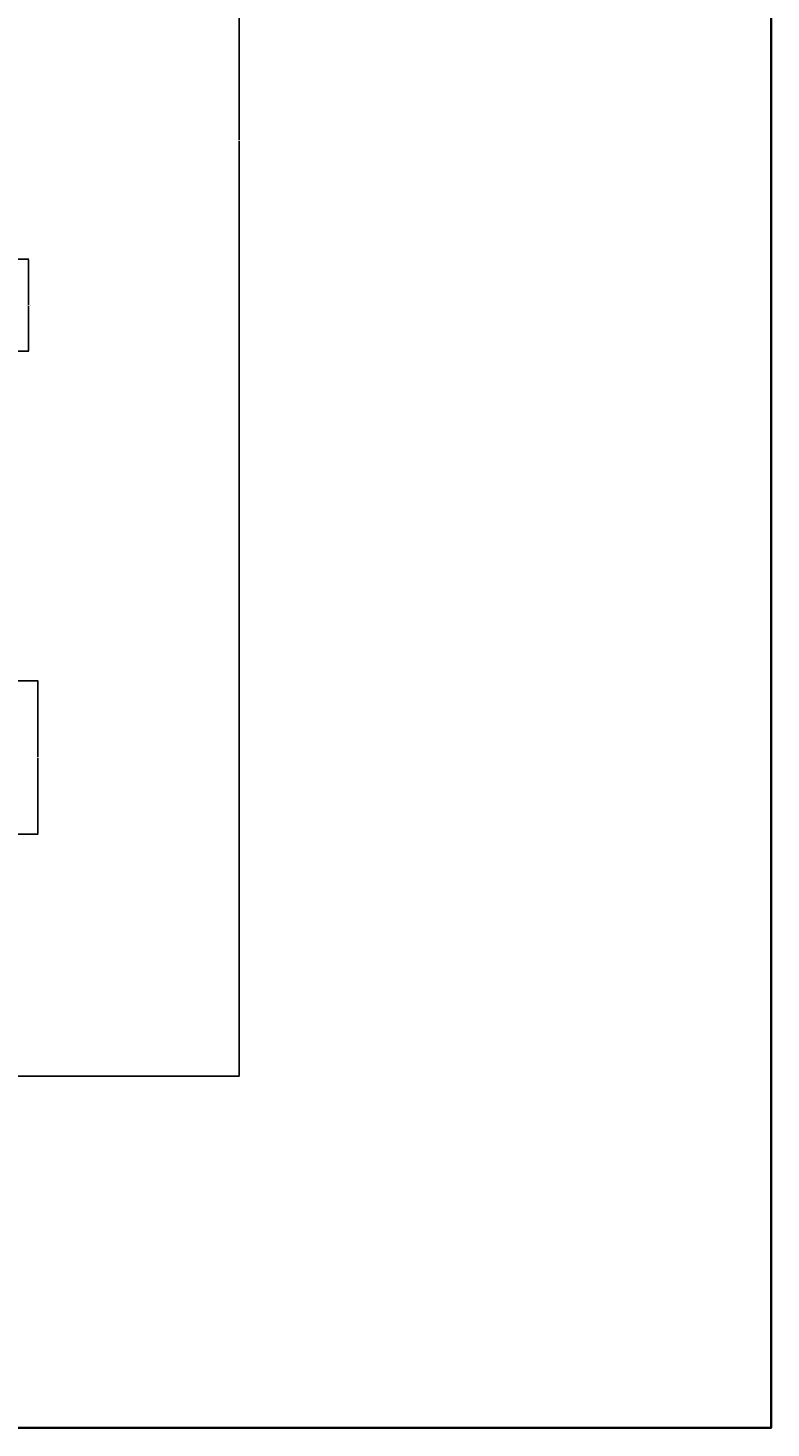
# Model space of a CAD drawing. Units: inches. Extents: x 1944 to 3454, y 1352 to 3055.
# Tile 12 of 17: x 3163 to 3454, y 1352 to 1900. Entities that reach past the tile are written whole.
import ezdxf

# ---------------------------------------------------------------- set-up
doc = ezdxf.new("R2010")
doc.units = ezdxf.units.IN
doc.layers.add('A-ANNO-DIMS', color=2, linetype='Continuous', lineweight=18)
doc.layers.add('A-ANNO-TTLB', color=7, linetype='Continuous', lineweight=35)
doc.styles.get("Standard").update_dxf_attribs({"font": 'arial.ttf'})
doc.dimstyles.get("Standard").update_dxf_attribs({"dimtxt": 0.18, "dimasz": 0.18, "dimexe": 0.18, "dimexo": 0.0625, "dimgap": 0.09, "dimtad": 0, "dimtih": 1, "dimtoh": 1, "dimdec": 4, "dimzin": 0, "dimdsep": 46, "dimtxsty": 'Standard', "dimcen": 0.09, "dimadec": 0, "dimazin": 0, "dimtfac": 1, "dimtdec": 4, "dimtofl": 0, "dimtmove": 0, "dimatfit": 3, "dimfxl": 1, "dimtolj": 1, "dimtzin": 0, "dimarcsym": 0})

# ---------------------------------------------------------------- blocks, each defined once
blk = doc.blocks.new('*D70')
at = {"layer": 'A-ANNO-DIMS', "color": 0, "lineweight": -2, "transparency": 16777216}
for p, q in [((3157.44, 1809.51), (3162.96, 1809.51)), ((3162.78, 1809.33), (3162.78, 1791.69)), ((3162.78, 1773.69), (3162.78, 1791.32)), ((3157.44, 1773.51), (3162.96, 1773.51))]:
    blk.add_line(p, q, dxfattribs=at)
at = {"layer": 'A-ANNO-DIMS', "color": 0, "transparency": 16777216}
for points in [[(3162.75, 1809.33), (3162.81, 1809.33), (3162.78, 1809.51)], [(3162.75, 1773.69), (3162.81, 1773.69), (3162.78, 1773.51)]]:
    blk.add_solid(points, dxfattribs=at)
at = {"layer": 'Defpoints', "color": 0, "transparency": 16777216}
for p in [(3157.38, 1809.51), (3162.78, 1809.51), (3157.38, 1773.51)]:
    blk.add_point(p, dxfattribs=at)
at = {"layer": 'A-ANNO-DIMS', "color": 0, "transparency": 16777216, "insert": (3162.78, 1791.51), "char_height": 0.18, "attachment_point": 5}
blk.add_mtext('\\A1;WINDOW 36 TYP.', dxfattribs=at)
blk = doc.blocks.new('*D78')
at = {"layer": 'A-ANNO-DIMS', "color": 0, "lineweight": -2, "transparency": 16777216}
for p, q in [((3157.44, 1644.39), (3166.56, 1644.39)), ((3166.38, 1644.21), (3166.38, 1614.57)), ((3166.38, 1584.57), (3166.38, 1614.21)), ((3157.44, 1584.39), (3166.56, 1584.39))]:
    blk.add_line(p, q, dxfattribs=at)
at = {"layer": 'A-ANNO-DIMS', "color": 0, "transparency": 16777216}
for points in [[(3166.35, 1644.21), (3166.41, 1644.21), (3166.38, 1644.39)], [(3166.35, 1584.57), (3166.41, 1584.57), (3166.38, 1584.39)]]:
    blk.add_solid(points, dxfattribs=at)
at = {"layer": 'Defpoints', "color": 0, "transparency": 16777216}
for p in [(3157.38, 1644.39), (3166.38, 1644.39), (3157.38, 1584.39)]:
    blk.add_point(p, dxfattribs=at)
at = {"layer": 'A-ANNO-DIMS', "color": 0, "transparency": 16777216, "insert": (3166.38, 1614.39), "char_height": 0.18, "attachment_point": 5}
blk.add_mtext('\\A1;WINDOW 60 TYP.', dxfattribs=at)
blk = doc.blocks.new('*D187')
at = {"layer": 'A-ANNO-DIMS', "color": 0, "lineweight": -2, "transparency": 16777216}
for p, q in [((3089.53, 2222.6), (3245.46, 2222.6)), ((3245.28, 2222.42), (3245.28, 1856.28)), ((3245.28, 1489.78), (3245.28, 1855.91)), ((3093.18, 1489.6), (3245.46, 1489.6))]:
    blk.add_line(p, q, dxfattribs=at)
at = {"layer": 'A-ANNO-DIMS', "color": 0, "transparency": 16777216}
for points in [[(3245.25, 2222.42), (3245.31, 2222.42), (3245.28, 2222.6)], [(3245.25, 1489.78), (3245.31, 1489.78), (3245.28, 1489.6)]]:
    blk.add_solid(points, dxfattribs=at)
at = {"layer": 'Defpoints', "color": 0, "transparency": 16777216}
for p in [(3089.47, 2222.6), (3245.28, 2222.6), (3093.12, 1489.6)]:
    blk.add_point(p, dxfattribs=at)
at = {"layer": 'A-ANNO-DIMS', "color": 0, "transparency": 16777216, "insert": (3245.28, 1856.1), "char_height": 0.18, "attachment_point": 5}
blk.add_mtext('\\A1;733', dxfattribs=at)

msp = doc.modelspace()

# ---------------------------------------------------------------- linework, layer by layer
at = {"layer": 'A-ANNO-TTLB'}
msp.add_lwpolyline([(1943.914, 3054.605), (3453.633, 3054.605), (3453.633, 1351.76), (1943.914, 1351.76)], close=True, dxfattribs=at)

# ---------------------------------------------------------------- dimensions: what is measured, and where the dimension line sits
at = {"layer": 'A-ANNO-DIMS'}
dim = msp.add_linear_dim(base=(3245.282, 2222.596), p1=(3093.12, 1489.596), p2=(3089.47, 2222.596), angle=90, dimstyle='Standard', override={"dimdec": 0, "dimlfac": 1, "dimrnd": 0, "dimzin": 0, "dimdsep": 46, "dimlunit": 2}, dxfattribs=at)
dim.commit()
dim.dimension.update_dxf_attribs({"geometry": '*D187', "text_midpoint": (3245.282, 1856.096)})
for base, p1, p2, picture, middle in [((3162.775, 1809.506), (3157.375, 1773.506), (3157.375, 1809.506), '*D70', (3162.775, 1791.506)), ((3166.375, 1644.389), (3157.375, 1584.389), (3157.375, 1644.389), '*D78', (3166.375, 1614.389))]:
    dim = msp.add_linear_dim(base=base, p1=p1, p2=p2, angle=90, text='WINDOW <> TYP.', dimstyle='Standard', override={"dimdec": 0, "dimlfac": 1, "dimrnd": 0, "dimzin": 0, "dimdsep": 46, "dimlunit": 2}, dxfattribs=at)
    dim.commit()
    dim.dimension.update_dxf_attribs({"geometry": picture, "text_midpoint": middle})

doc.saveas('drawing.dxf')
